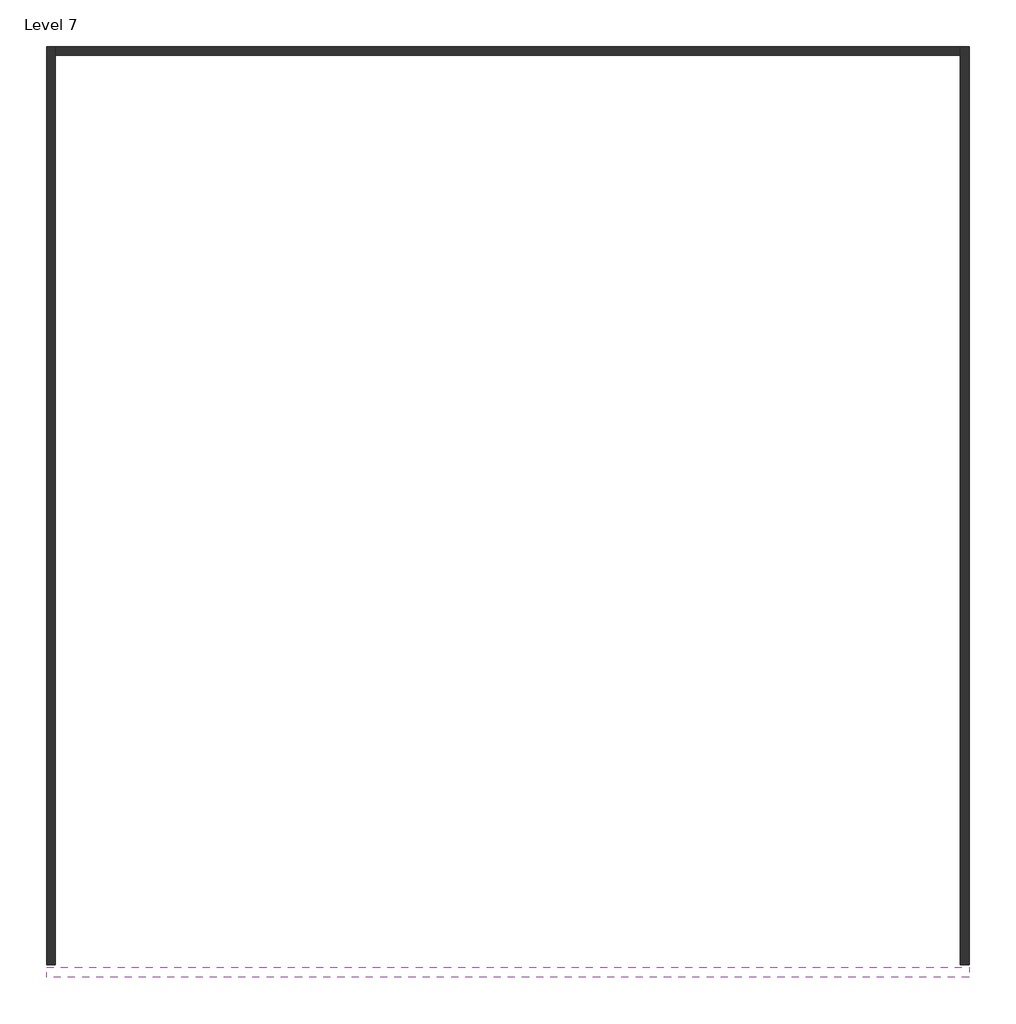
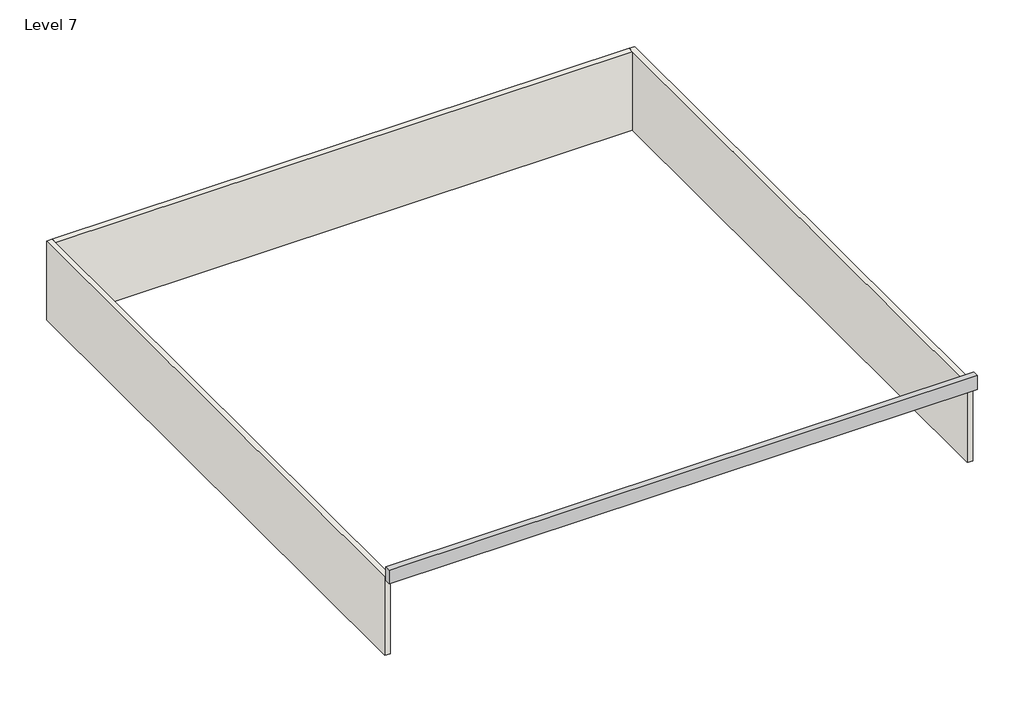
# One storey: 3 walls, 1 proxy.
"""IFC4 building model written with IfcOpenShell, lengths in millimetres."""

from ifc_helpers import new_model, si_unit, frame, origin, place, context, project, spatial, polyline, outline, extrude, faceted_brep, transform, mapped, element, save
from components import generic_models_6_generic_models_6_95f07958

model = new_model("IFC4")

# Units and contexts
model_context = context("Model", 3, world=origin())
ifc_project = project(units=[si_unit("LENGTHUNIT", "METRE", prefix="MILLI")], contexts=[model_context])

# Site, building, storey
site = spatial("IfcSite", under=ifc_project)
building = spatial("IfcBuilding", under=site)
storey = spatial("IfcBuildingStorey", under=building, Name="Level 7", Elevation=9829.8)

# Proxy
placement = place(None, origin())
generic_models_6_generic_models_6_shape = generic_models_6_generic_models_6_95f07958(model_context)
element("IfcBuildingElementProxy", 1, Name="Generic Models 6 : Generic Models 6", ObjectType="Generic Models 6 : Generic Models 6", at=placement, inside=storey, context=model_context, shape_type="MappedRepresentation", body=[
    mapped(generic_models_6_generic_models_6_shape, transform((0.0, 0.0, 0.0), x_axis=(1.0, 0.0, 0.0), y_axis=(0.0, 1.0, 0.0), z_axis=(0.0, 0.0, 1.0))),
])

# Walls
element("IfcWall", 2, ObjectType="outer wall", at=placement, inside=storey, context=model_context, shape_type="Brep", body=[
    faceted_brep([(-8731.5629849, -3682.5004242, 9829.8), (-8731.5629849, 17551.8995758, 9829.8), (-8731.5629849, 17755.0995758, 9829.8), (-8731.5629849, 17755.0995758, 12877.8), (-8731.5629849, 17551.8995758, 12877.8), (-8731.5629849, -3682.5004242, 12877.8), (-8934.7629849, -3682.5004242, 9829.8), (-8934.7629849, -3682.5004242, 12877.8), (-8934.7629849, 17755.0995758, 12877.8), (-8934.7629849, 17755.0995758, 9829.8)], [[[0, 1, 2, 3, 4, 5]], [[6, 7, 8, 9]], [[2, 1, 0, 6, 9]], [[0, 5, 7, 6]], [[5, 4, 3, 8, 7]], [[3, 2, 9, 8]]]),
])
element("IfcWall", 3, ObjectType="outer wall", at=placement, inside=storey, context=model_context, shape_type="Brep", body=[
    faceted_brep([(12401.2370151, 17755.0995758, 9829.8), (12401.2370151, 17551.8995758, 9829.8), (12401.2370151, -3682.5004242, 9829.8), (12401.2370151, -3682.5004242, 12877.8), (12401.2370151, 17551.8995758, 12877.8), (12401.2370151, 17755.0995758, 12877.8), (12604.4370151, 17755.0995758, 9829.8), (12604.4370151, 17755.0995758, 12877.8), (12604.4370151, -3682.5004242, 12877.8), (12604.4370151, -3682.5004242, 9829.8)], [[[0, 1, 2, 3, 4, 5]], [[6, 7, 8, 9]], [[2, 1, 0, 6, 9]], [[3, 2, 9, 8]], [[5, 4, 3, 8, 7]], [[0, 5, 7, 6]]]),
])
element("IfcWall", 4, ObjectType="outer wall", at=placement, inside=storey, context=model_context, shape_type="SweptSolid", body=[
    extrude(outline(polyline([(12401.2370151, 17551.8995758), (-8731.5629849, 17551.8995758), (-8731.5629849, 17755.0995758), (12401.2370151, 17755.0995758), (12401.2370151, 17551.8995758)])), frame((0.0, 0.0, 9829.8), z_axis=(0.0, 0.0, 1.0), x_axis=(1.0, 0.0, 0.0)), (0.0, 0.0, 1.0), 3048.0),
])

save(model, "model.ifc")

# Revit data of these elements
# Type "outer wall"
#   Assembly Code = "B2010"
#   Layers, outside or top first: 0' - 8" "Copper" (function 1)
# Element 1 (IfcBuildingElementProxy, "Generic Models 6 : Generic Models 6")
#   Phase Created = New Construction
# Elements 2, 3, 4 (IfcWall, "outer wall")
#   Top Offset = 0' - 0"
#   Base Offset = 0' - 0"
#   Unconnected Height = 10' - 0"
#   wall height = 10' - 0"
#   Phase Created = New Construction
#   Base Constraint = Level 7
#   Materials on its faces: "Copper"
# Materials
#   "Copper": class "Metal", colour RGB 0 0 0, transparency 0, Description = "Copper, matte finish", Cost = 0
